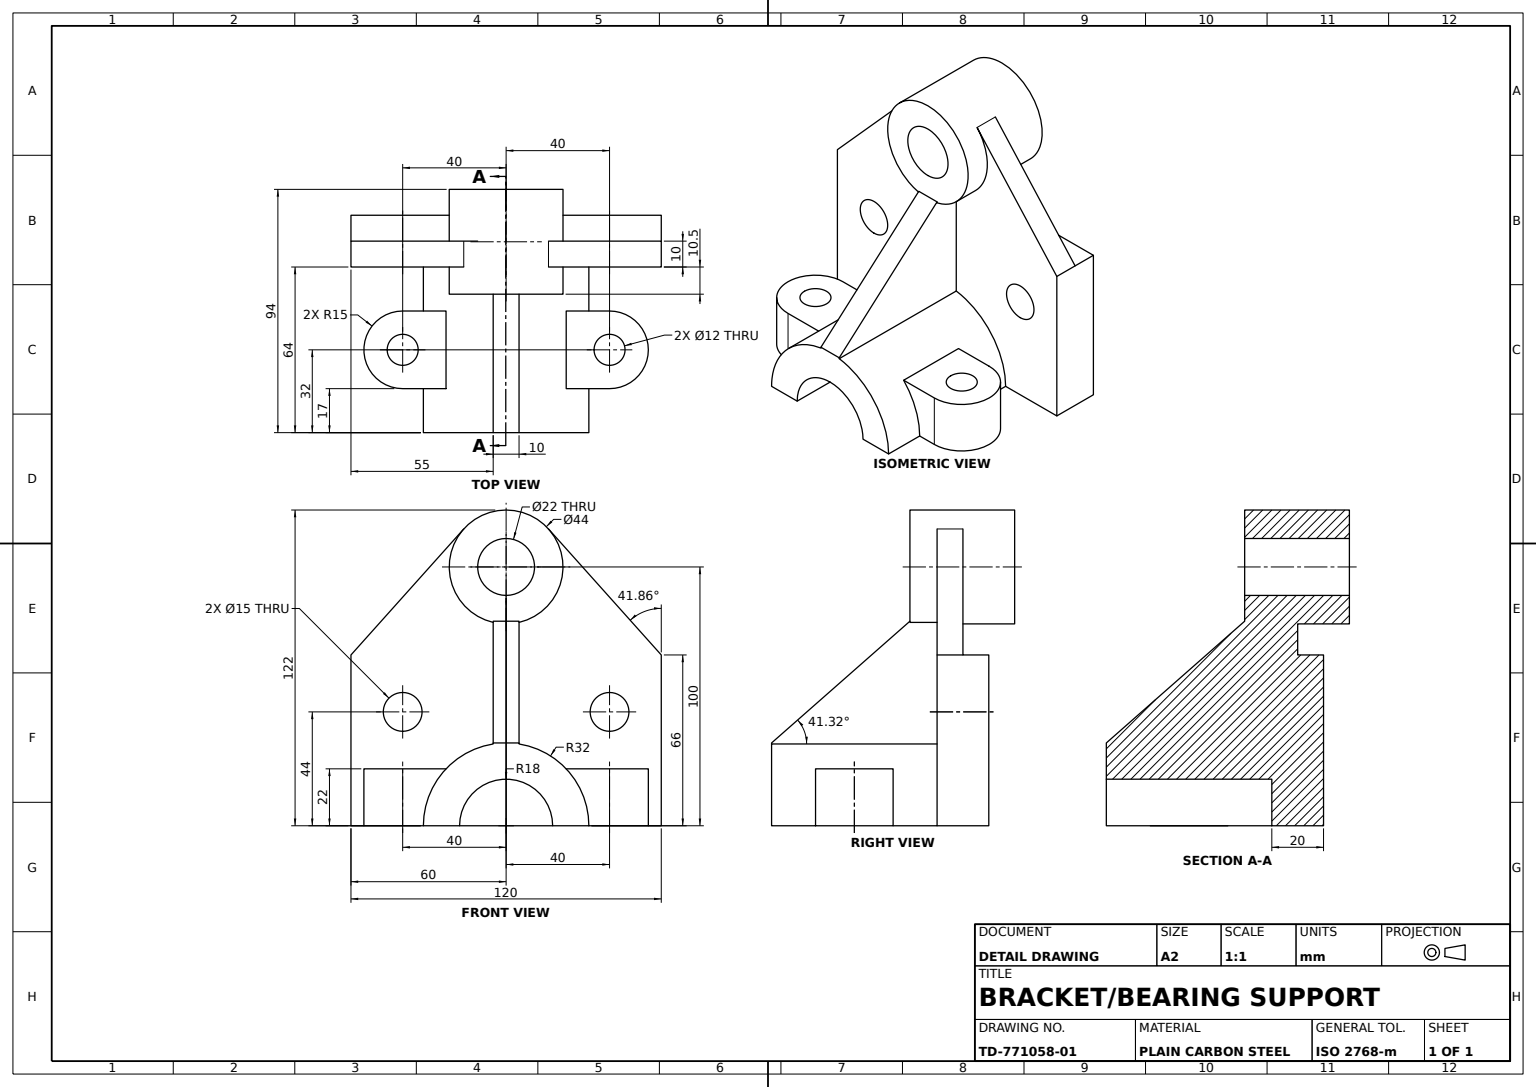
from build123d import *
from build123d.topology import SkipClean

# Parameters (mm, degrees)
BASE_PLATE_SKETCH_W            = 20
BASE_PLATE_SKETCH_H            = 66
BASE_PLATE_DEPTH               = 120
UPRIGHT_WEB_SKETCH_R           = 22
UPRIGHT_WEB_SKETCH_R_2         = 11
UPRIGHT_WEB_DEPTH              = 10
TRUNNION_BOSS_FRONT_SKETCH_R   = 22
TRUNNION_BOSS_FRONT_SKETCH_R_2 = 11
TRUNNION_BOSS_FRONT_DEPTH      = 20
TRUNNION_START                 = 10
TRUNNION_BOSS_REAR_SKETCH_R    = 22
TRUNNION_BOSS_REAR_SKETCH_R_2  = 11
TRUNNION_BOSS_REAR_DEPTH       = 10
BRACKET_HOLES_SKETCH_R         = 7.5
BRACKET_HOLES_DEPTH            = 30
SEMI_CIRCULAR_BASE_DEPTH       = 64
GUSSET_1_DEPTH                 = 5
GUSSET_START                   = -64
GUSSET_2_DEPTH                 = 64
TRUNNION_START_2               = 0.5
TRUNNION_FACE_PAD_SKETCH_R     = 22
TRUNNION_FACE_PAD_SKETCH_R_2   = 11
TRUNNION_FACE_PAD_0_5MM_DEPTH  = 0.5
BASE_MOUNTING_LUGS_SKETCH_R    = 6
BASE_MOUNTING_LUGS_DEPTH       = 22


with BuildPart() as part:
    # Base Plate Sketch → Base Plate (new body)
    with BuildSketch(Plane.XY):
        Rectangle(BASE_PLATE_SKETCH_W, BASE_PLATE_SKETCH_H)
    extrude(amount=BASE_PLATE_DEPTH)

    # Upright Web Sketch → Upright Web (add)
    # profile 1 of 2: a face of its own
    with BuildSketch(Plane(origin=(10, 0, 0), x_dir=(0, 0, -1), z_dir=(1, 0, 0))):
        with BuildLine():
            Line((-76.38555148, 81.680384964), (-120, 33))
            Line((-120, 33), (0, 33))
            Line((0, 33), (-43.61444852, 81.680384964))
            ThreePointArc((-43.61444852, 81.680384964), (-39.451494792, 74.858685241), (-38, 67))
            ThreePointArc((-38, 67), (-67.858685241, 46.451494792), (-76.38555148, 81.680384964))
        make_face()
    # profile 2 of 2: a face of its own
    with BuildSketch(Plane(origin=(10, 0, 0), x_dir=(0, 0, -1), z_dir=(1, 0, 0))):
        with Locations((-60, 67)):
            Circle(UPRIGHT_WEB_SKETCH_R)
        with Locations(Location((-60, 67, 0), (0, 0, 90))):
            Circle(UPRIGHT_WEB_SKETCH_R_2, mode=Mode.SUBTRACT)
    extrude(amount=-UPRIGHT_WEB_DEPTH)

    # Trunnion Boss Front Sketch → Trunnion Boss Front (add)
    with SkipClean():  # the faces are left unmerged after this step: merging them gives an invalid solid
        with BuildSketch(Plane.ZY):
            with Locations(Location((60, 67, 0), (0, 0, 41.858266049))):
                Circle(TRUNNION_BOSS_FRONT_SKETCH_R)
            with Locations(Location((60, 67, 0), (0, 0, 90))):
                Circle(TRUNNION_BOSS_FRONT_SKETCH_R_2, mode=Mode.SUBTRACT)
        extrude(amount=TRUNNION_BOSS_FRONT_DEPTH)

    # Trunnion Boss Rear Sketch → Trunnion Boss Rear (add)
    with SkipClean():  # the faces are left unmerged after this step: merging them gives an invalid solid
        with BuildSketch(Plane(origin=(10, 0, 0), x_dir=(0, 0, -1), z_dir=(1, 0, 0)).offset(TRUNNION_START)):
            with Locations(Location((-60, 67, 0), (0, 0, 90))):
                Circle(TRUNNION_BOSS_REAR_SKETCH_R)
            with Locations(Location((-60, 67, 0), (0, 0, 90))):
                Circle(TRUNNION_BOSS_REAR_SKETCH_R_2, mode=Mode.SUBTRACT)
        extrude(amount=-TRUNNION_BOSS_REAR_DEPTH)

    # Bracket Holes Sketch → Bracket Holes (cut)
    with SkipClean():  # the faces are left unmerged after this step: merging them gives an invalid solid
        with BuildSketch(Plane(origin=(10, 0, 0), x_dir=(0, 0, -1), z_dir=(1, 0, 0))):
            with Locations(Location((-100, 11, 0), (0, 0, 90))):
                Circle(BRACKET_HOLES_SKETCH_R)
            with Locations(Location((-20, 11, 0), (0, 0, 90))):
                Circle(BRACKET_HOLES_SKETCH_R)
        extrude(amount=-BRACKET_HOLES_DEPTH, mode=Mode.SUBTRACT)

    # Semi-Circular Base Sketch → Semi-Circular Base (add)
    with SkipClean():  # the faces are left unmerged after this step: merging them gives an invalid solid
        with BuildSketch(Plane(origin=(10, 0, 0), x_dir=(0, 0, -1), z_dir=(1, 0, 0))):
            with BuildLine():
                Line((-92, -33), (-78, -33))
                ThreePointArc((-78, -33), (-60, -15), (-42, -33))
                Line((-42, -33), (-28, -33))
                ThreePointArc((-28, -33), (-60, -1), (-92, -33))
            make_face()
        extrude(amount=SEMI_CIRCULAR_BASE_DEPTH)



with BuildPart() as body_2:
    # Gusset 1 Sketch → Gusset 1 (new, symmetric)
    with BuildSketch(Plane.XY.offset(60)):
        Polygon((10, -5), (10, 46.478793063), (20, 46.478793063), (74, -1), (74, -5), align=None)
    extrude(amount=GUSSET_1_DEPTH, both=True)


with BuildPart() as part_1:
    with SkipClean():  # the faces are left unmerged after this step: merging them gives an invalid solid
        add(part.part)

        add(body_2.part)  # Gusset 2 merges body 2
        # Gusset 2 Sketch → Gusset 2 (add)
        with BuildSketch(Plane(origin=(74, 0, 0), x_dir=(0, 0, -1), z_dir=(1, 0, 0)).offset(GUSSET_START)):
            with BuildLine():
                Line((-92, -33), (-78, -33))
                ThreePointArc((-78, -33), (-60, -15), (-42, -33))
                Line((-42, -33), (-28, -33))
                ThreePointArc((-28, -33), (-60, -1), (-92, -33))
            make_face()
        extrude(amount=GUSSET_2_DEPTH)

    # Trunnion Face Pad Sketch → Trunnion Face Pad 0.5mm (add)
    with SkipClean():  # the faces are left unmerged after this step: merging them gives an invalid solid
        with BuildSketch(Plane(origin=(20, 0, 0), x_dir=(0, 0, -1), z_dir=(1, 0, 0)).offset(TRUNNION_START_2)):
            with Locations(Location((-60, 67, 0), (0, 0, 138.141733951))):
                Circle(TRUNNION_FACE_PAD_SKETCH_R)
            with Locations(Location((-60, 67, 0), (0, 0, 90))):
                Circle(TRUNNION_FACE_PAD_SKETCH_R_2, mode=Mode.SUBTRACT)
        extrude(amount=-TRUNNION_FACE_PAD_0_5MM_DEPTH)

    # Base Mounting Lugs Sketch → Base Mounting Lugs (add)
    # profile 1 of 2: a face of its own
    with SkipClean():  # the faces are left unmerged after this step: merging them gives an invalid solid
        with BuildSketch(Plane.XZ.offset(33)):
            with BuildLine():
                Line((27, 100), (27, 83))
                Line((27, 83), (57, 83))
                Line((57, 83), (57, 85))
                Line((57, 85), (57, 100))
                ThreePointArc((57, 100), (42, 115), (27, 100))
            make_face()
            with Locations(Location((42, 100, 0), (0, 0, 270))):
                Circle(BASE_MOUNTING_LUGS_SKETCH_R, mode=Mode.SUBTRACT)
        # profile 2 of 2: a face of its own
        with BuildSketch(Plane.XZ.offset(33)):
            with BuildLine():
                Line((27, 20), (27, 38))
                Line((27, 38), (57, 38))
                Line((57, 38), (57, 35))
                Line((57, 35), (57, 20))
                ThreePointArc((57, 20), (42, 5), (27, 20))
            make_face()
            with Locations(Location((42, 20, 0), (0, 0, 270))):
                Circle(BASE_MOUNTING_LUGS_SKETCH_R, mode=Mode.SUBTRACT)
        extrude(amount=-BASE_MOUNTING_LUGS_DEPTH)


solid = part_1.part
